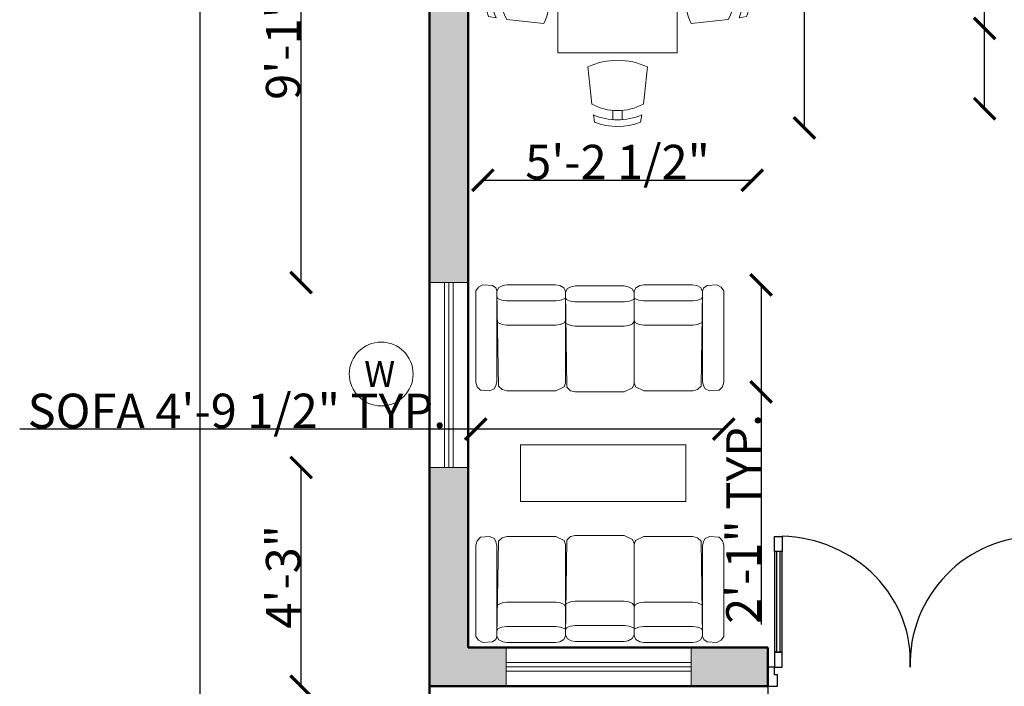
# Model space of a CAD drawing. Units: inches. Extents: x 2169 to 2662, y 1518 to 2151.
# Tile 2 of 6: x 2169 to 2398, y 1596 to 1751. Entities that reach past the tile are written whole.
import ezdxf

# ---------------------------------------------------------------- set-up
doc = ezdxf.new("R2010")
doc.units = ezdxf.units.IN
for name, color, linetype, lineweight in [('A-ANNO-DIMS', 2, 'Continuous', 18), ('A-ANNO-SYMB', 7, 'Continuous', 18), ('A-FURN', 8, 'Continuous', 18), ('A-WALL-PATT', 30, 'Continuous', 13), ('L-PLNT-BEDS', 94, 'Continuous', 25), ('Main Door', 150, 'Continuous', 30), ('Walls', 7, 'Continuous', 50), ('Windows', 160, 'Continuous', 18)]:
    doc.layers.add(name, color=color, linetype=linetype, lineweight=lineweight)
doc.layers.add('A-Glaz', color=92, linetype='Continuous')
doc.styles.get("Standard").update_dxf_attribs({"font": 'arial.ttf'})
doc.dimstyles.get("Standard").update_dxf_attribs({"dimtxt": 8, "dimasz": 5, "dimexe": 0.18, "dimexo": 0.0625, "dimgap": 0.09, "dimtad": 1, "dimdec": 1, "dimzin": 0, "dimdsep": 46, "dimlunit": 4, "dimtxsty": 'Standard', "dimblk": 'ARCHTICK', "dimcen": 0.09, "dimse1": 1, "dimse2": 1, "dimadec": 0, "dimazin": 0, "dimtfac": 1, "dimtdec": 1, "dimtofl": 0, "dimtmove": 0, "dimatfit": 3, "dimfxl": 1, "dimtolj": 1, "dimtzin": 0, "dimarcsym": 0})

# ---------------------------------------------------------------- blocks, each defined once
blk = doc.blocks.new('_ArchTick')
at = {"color": 0, "linetype": 'ByBlock', "const_width": 0.15}
blk.add_lwpolyline([(-0.5, -0.5), (0.5, 0.5)], dxfattribs=at)
blk = doc.blocks.new('*D4')
at = {"layer": 'A-ANNO-DIMS', "color": 0, "lineweight": -2, "transparency": 16777216}
blk.add_line((2210.62, 1555.6), (2210.62, 2111.6), dxfattribs=at)
at = {"layer": 'Defpoints', "color": 0, "transparency": 16777216}
for p in [(2210.62, 2111.6), (2263.98, 2111.6), (2263.98, 1555.6)]:
    blk.add_point(p, dxfattribs=at)
at = {"layer": 'A-ANNO-DIMS', "color": 0, "lineweight": -2, "transparency": 16777216, "xscale": 5, "yscale": 5, "zscale": 5}
for p, rotation in [((2210.62, 2111.6), 90), ((2210.62, 1555.6), 270)]:
    blk.add_blockref('_ArchTick', p, dxfattribs=dict(at, rotation=rotation))
at = {"layer": 'A-ANNO-DIMS', "color": 0, "transparency": 16777216, "insert": (2206.45, 1833.6), "char_height": 8, "attachment_point": 5, "rotation": 90}
blk.add_mtext('\\A1;46\'-4"', dxfattribs=at)
blk = doc.blocks.new('A$C13CE0A17')
at = {"layer": 'A-Glaz'}
for p, q in [((0.01, 0.61), (0.01, 0.08)), ((0.03, 0.08), (0.03, 0.61))]:
    blk.add_line(p, q, dxfattribs=at)
blk.add_lwpolyline([(1.4, 0.08), (1.4, 0.61), (1.42, 0.61), (1.42, 0.08)], close=True, dxfattribs=at)
at = {"layer": 'Main Door'}
for p, q in [((0, 0.61), (0, 0.69)), ((0, 0.69), (0.04, 0.69)), ((0.04, 0.69), (0.04, 0.61)), ((0, 0.61), (0, 0.08)), ((0.04, 0.61), (0, 0.61)), ((0.04, 0.61), (0, 0.61)), ((0.03, 0.61), (0.01, 0.61)), ((0.04, 0.08), (0.04, 0.61)), ((0, 0.08), (0, 0)), ((0.04, 0.08), (0, 0.08)), ((0, 0.08), (0.04, 0.08)), ((0.01, 0.08), (0.03, 0.08)), ((0.04, 0), (0.04, 0.08)), ((-0.035, 0), (-0.035, -0.1)), ((0, 0), (-0.035, 0)), ((0, 0), (0.04, 0)), ((0, -0.04), (0, 0)), ((0.015, -0.04), (0, -0.04)), ((0.015, -0.05), (0.015, -0.04)), ((0.015, -0.1), (0.015, -0.05)), ((-0.035, -0.1), (0.015, -0.1))]:
    blk.add_line(p, q, dxfattribs=at)
for points in [[(1.39, 0.69), (1.39, 0.61), (1.43, 0.61), (1.43, 0.69)], [(1.39, 0.08), (1.39, 0.61), (1.43, 0.61), (1.43, 0.08)], [(1.39, 0), (1.39, 0.08), (1.43, 0.08), (1.43, 0)], [(1.43, 0), (1.465, 0), (1.465, -0.1), (1.415, -0.1), (1.415, -0.05), (1.415, -0.04), (1.43, -0.04)]]:
    blk.add_lwpolyline(points, close=True, dxfattribs=at)
blk.add_arc((1.3872, 0.017), 0.673, 89.7657, 181.4438, dxfattribs=at)
blk.add_ellipse((0.0389, 0.0511), major_axis=(0.6669, -0.1217), ratio=0.940794, start_param=0.11153, end_param=1.73917, dxfattribs=at)
blk = doc.blocks.new('12PCOU17')
at = {"color": 0, "linetype": 'ByBlock'}
for points in [[(-34.71, 34.72), (-33.66, 34.31), (-3.27, 34.3), (-1.81, 34.76), (-1.05, 35.2), (-0.38, 36.65), (-0.61, 39.84), (-1.73, 40.94), (-3.27, 41.4), (-33.66, 41.4), (-34.95, 40.5), (-35.65, 39.02), (-35.49, 35.83), (-34.71, 34.72)], [(-1.89, 11.91), (-1.66, 11.91), (-0.35, 14.68), (-0.35, 31.05), (-0.74, 32.58), (-1.89, 33.83), (-33.63, 34.3), (-34.84, 33.63), (-35.43, 32.38), (-35.68, 31), (-35.68, 14.74), (-35.43, 13.36), (-34.66, 11.99), (-33.44, 11.43), (-3, 11.44), (-1.66, 11.91)], [(-31.25, 11.43), (-31.06, 11.84), (-30.6, 13.09), (-30.4, 14.62), (-30.4, 31.12), (-30.6, 32.65), (-31.06, 33.9), (-31.81, 34.3)], [(-23.84, 11.43), (-22.99, 11.9), (-22.46, 13.15), (-22.23, 14.67), (-22.23, 31.07), (-22.46, 32.59), (-22.99, 33.84), (-23.12, 34.3)], [(-1.54, -10.96), (-1.31, -10.96), (0, -8.19), (0, 8.19), (-0.39, 9.71), (-1.54, 10.96), (-33.28, 11.44), (-34.5, 10.77), (-35.08, 9.51), (-35.33, 8.14), (-35.33, -8.13), (-35.08, -9.51), (-34.31, -10.87), (-33.1, -11.44), (-2.65, -11.43), (-1.31, -10.96)], [(-30.9, -11.44), (-30.72, -11.02), (-30.25, -9.77), (-30.05, -8.25), (-30.05, 8.26), (-30.25, 9.78), (-30.72, 11.03), (-31.47, 11.44)], [(-23.49, -11.44), (-22.64, -10.96), (-22.11, -9.72), (-21.88, -8.19), (-21.88, 8.2), (-22.11, 9.73), (-22.64, 10.97), (-22.77, 11.44)], [(-1.89, -11.91), (-1.66, -11.91), (-0.35, -14.68), (-0.35, -31.05), (-0.74, -32.58), (-1.89, -33.83), (-33.63, -34.3), (-34.84, -33.63), (-35.43, -32.38), (-35.68, -31), (-35.68, -14.74), (-35.43, -13.36), (-34.66, -11.99), (-33.44, -11.43), (-3, -11.44), (-1.66, -11.91)], [(-31.25, -11.43), (-31.06, -11.84), (-30.6, -13.09), (-30.4, -14.62), (-30.4, -31.12), (-30.6, -32.65), (-31.06, -33.9), (-31.81, -34.3)], [(-23.84, -11.43), (-22.99, -11.9), (-22.46, -13.15), (-22.23, -14.67), (-22.23, -31.07), (-22.46, -32.59), (-22.99, -33.84), (-23.12, -34.3)], [(-34.71, -34.72), (-33.66, -34.31), (-3.27, -34.3), (-1.81, -34.76), (-1.05, -35.2), (-0.38, -36.65), (-0.61, -39.84), (-1.73, -40.94), (-3.27, -41.4), (-33.66, -41.4), (-34.95, -40.5), (-35.65, -39.02), (-35.49, -35.83), (-34.71, -34.72)]]:
    blk.add_lwpolyline(points, dxfattribs=at)
blk = doc.blocks.new('table-23')
at = {"color": 0, "linetype": 'ByBlock'}
for p, q in [((-0.6323, 0.4685), (-0.6236, 0.5245)), ((-0.2677, 0.4685), (-0.2764, 0.5245)), ((-0.485, 0.5057), (-0.485, 0.4355)), ((-0.415, 0.5057), (-0.415, 0.4355)), ((-0.675, 0.107), (-0.645, 0.387)), ((-0.225, 0.107), (-0.255, 0.387)), ((-0.9, -1.4923), (-0.9, 0)), ((-0.9, 0), (0, 0)), ((0, -1.4923), (0, 0)), ((-1.0062, -0.2211), (-1.2862, -0.2511)), ((0.1062, -0.2211), (0.3862, -0.2511)), ((-1.3677, -0.2639), (-1.4237, -0.2726)), ((0.4677, -0.2639), (0.5237, -0.2726)), ((-1.4049, -0.4111), (-1.3347, -0.4111)), ((0.5049, -0.4111), (0.4347, -0.4111)), ((-1.4049, -0.4811), (-1.3347, -0.4811)), ((0.5049, -0.4811), (0.4347, -0.4811)), ((-1.3677, -0.6284), (-1.4237, -0.6197)), ((-1.0062, -0.6711), (-1.2862, -0.6411)), ((0.1062, -0.6711), (0.3862, -0.6411)), ((0.4677, -0.6284), (0.5237, -0.6197)), ((-1.3677, -0.8639), (-1.4237, -0.8726)), ((-1.0062, -0.8211), (-1.2862, -0.8511)), ((0.1062, -0.8211), (0.3862, -0.8511)), ((0.4677, -0.8639), (0.5237, -0.8726)), ((-1.4049, -1.0111), (-1.3347, -1.0111)), ((0.5049, -1.0111), (0.4347, -1.0111)), ((-1.4049, -1.0811), (-1.3347, -1.0811)), ((0.5049, -1.0811), (0.4347, -1.0811)), ((-1.3677, -1.2284), (-1.4237, -1.2197)), ((-1.0062, -1.2711), (-1.2862, -1.2411)), ((0.1062, -1.2711), (0.3862, -1.2411)), ((0.4677, -1.2284), (0.5237, -1.2197)), ((-0.9, -1.4923), (0, -1.4923)), ((-0.675, -1.5993), (-0.645, -1.8793)), ((-0.225, -1.5993), (-0.255, -1.8793)), ((-0.485, -1.998), (-0.485, -1.9278)), ((-0.415, -1.998), (-0.415, -1.9278)), ((-0.6323, -1.9608), (-0.6236, -2.0168)), ((-0.2677, -1.9608), (-0.2764, -2.0168))]:
    blk.add_line(p, q, dxfattribs=at)
for centre, radius, start, end in [((-0.45, 0.0773), 0.4797, 68.78869, 111.21131), ((-0.45, 0.0566), 0.4505, 66.13443, 113.86557), ((-0.45, 0.0318), 0.4053, 61.23721, 118.76279), ((-0.45, 0.5883), 0.5312, 244.94238, 295.05762), ((-1.4875, -0.4461), 0.5312, 334.94238, 25.05762), ((0.5875, -0.4461), 0.5312, 154.94238, 205.05762), ((-0.9765, -0.4461), 0.4797, 158.78869, 201.21131), ((-0.9558, -0.4461), 0.4505, 156.13443, 203.86557), ((-0.931, -0.4461), 0.4053, 151.23721, 208.76279), ((0.031, -0.4461), 0.4053, 331.23721, 28.76279), ((0.0558, -0.4461), 0.4505, 336.13443, 23.86557), ((0.0765, -0.4461), 0.4797, 338.78869, 21.21131), ((-0.9765, -1.0461), 0.4797, 158.78869, 201.21131), ((-0.9558, -1.0461), 0.4505, 156.13443, 203.86557), ((-0.931, -1.0461), 0.4053, 151.23721, 208.76279), ((-1.4875, -1.0461), 0.5312, 334.94238, 25.05762), ((0.5875, -1.0461), 0.5312, 154.94238, 205.05762), ((0.031, -1.0461), 0.4053, 331.23721, 28.76279), ((0.0558, -1.0461), 0.4505, 336.13443, 23.86557), ((0.0765, -1.0461), 0.4797, 338.78869, 21.21131), ((-0.45, -2.0806), 0.5312, 64.94238, 115.05762), ((-0.45, -1.5241), 0.4053, 241.23721, 298.76279), ((-0.45, -1.5489), 0.4505, 246.13443, 293.86557), ((-0.45, -1.5696), 0.4797, 248.78869, 291.21131)]:
    blk.add_arc(centre, radius, start, end, dxfattribs=at)
blk = doc.blocks.new('GLAZING-43IN')
for p, q in [((-21.5, 1), (21.5, 1)), ((-21.5, 0), (21.5, 0)), ((-21.5, -1), (21.5, -1))]:
    blk.add_line(p, q)
blk = doc.blocks.new('OPENING-TAG-W')
blk.add_circle((0, 0), 7.42)
blk.add_text('W', height=6).set_placement((-3.96, -3))
blk = doc.blocks.new('*D41')
at = {"layer": 'A-ANNO-DIMS', "color": 0, "lineweight": -2, "transparency": 16777216}
for p, q in [((2342.72, 1585.67), (2408.92, 1585.67)), ((2408.92, 1585.67), (2502.68, 1585.67))]:
    blk.add_line(p, q, dxfattribs=at)
at = {"layer": 'Defpoints', "color": 0, "transparency": 16777216}
for p in [(2342.72, 1595.6), (2408.92, 1595.6), (2408.92, 1585.67)]:
    blk.add_point(p, dxfattribs=at)
at = {"layer": 'A-ANNO-DIMS', "color": 0, "lineweight": -2, "transparency": 16777216, "xscale": 5, "yscale": 5, "zscale": 5, "rotation": 180}
blk.add_blockref('_ArchTick', (2342.72, 1585.67), dxfattribs=at)
at = {"layer": 'A-ANNO-DIMS', "color": 0, "lineweight": -2, "transparency": 16777216, "xscale": 5, "yscale": 5, "zscale": 5}
blk.add_blockref('_ArchTick', (2408.92, 1585.67), dxfattribs=at)
at = {"layer": 'A-ANNO-DIMS', "color": 0, "transparency": 16777216, "insert": (2458.3, 1589.9), "char_height": 8, "attachment_point": 5}
blk.add_mtext('\\A1;MAIN DOOR 5\'-6"', dxfattribs=at)
blk = doc.blocks.new('*D45')
at = {"layer": 'A-ANNO-DIMS', "color": 0, "lineweight": -2, "transparency": 16777216}
for p, q in [((2274.75, 1655.41), (2168.67, 1655.41)), ((2332.47, 1655.41), (2274.75, 1655.41))]:
    blk.add_line(p, q, dxfattribs=at)
at = {"layer": 'Defpoints', "color": 0, "transparency": 16777216}
for p in [(2274.75, 1664.07), (2332.47, 1664.07), (2274.75, 1655.41)]:
    blk.add_point(p, dxfattribs=at)
at = {"layer": 'A-ANNO-DIMS', "color": 0, "lineweight": -2, "transparency": 16777216, "xscale": 5, "yscale": 5, "zscale": 5, "rotation": 180}
blk.add_blockref('_ArchTick', (2274.75, 1655.41), dxfattribs=at)
at = {"layer": 'A-ANNO-DIMS', "color": 0, "lineweight": -2, "transparency": 16777216, "xscale": 5, "yscale": 5, "zscale": 5}
blk.add_blockref('_ArchTick', (2332.47, 1655.41), dxfattribs=at)
at = {"layer": 'A-ANNO-DIMS', "color": 0, "transparency": 16777216, "insert": (2219.21, 1659.64), "char_height": 8, "attachment_point": 5}
blk.add_mtext('\\A1;SOFA 4\'-9 1/2" TYP.', dxfattribs=at)
blk = doc.blocks.new('*D46')
at = {"layer": 'A-ANNO-DIMS', "color": 0, "lineweight": -2, "transparency": 16777216}
for p, q in [((2341.13, 1688.94), (2341.13, 1664.07)), ((2341.13, 1664.07), (2341.13, 1609.99))]:
    blk.add_line(p, q, dxfattribs=at)
at = {"layer": 'Defpoints', "color": 0, "transparency": 16777216}
for p in [(2332.47, 1688.94), (2332.47, 1664.07), (2341.13, 1664.07)]:
    blk.add_point(p, dxfattribs=at)
at = {"layer": 'A-ANNO-DIMS', "color": 0, "lineweight": -2, "transparency": 16777216, "xscale": 5, "yscale": 5, "zscale": 5}
for p, rotation in [((2341.13, 1688.94), 90), ((2341.13, 1664.07), 270)]:
    blk.add_blockref('_ArchTick', p, dxfattribs=dict(at, rotation=rotation))
at = {"layer": 'A-ANNO-DIMS', "color": 0, "transparency": 16777216, "insert": (2337.02, 1634.53), "char_height": 8, "attachment_point": 5, "rotation": 90}
blk.add_mtext('\\A1;2\'-1" TYP.', dxfattribs=at)
blk = doc.blocks.new('*D47')
at = {"layer": 'A-ANNO-DIMS', "color": 0, "lineweight": -2, "transparency": 16777216}
for p, q in [((2351.22, 1806.38), (2351.22, 1899.49)), ((2351.22, 1725.43), (2351.22, 1806.38))]:
    blk.add_line(p, q, dxfattribs=at)
at = {"layer": 'Defpoints', "color": 0, "transparency": 16777216}
for p in [(2339.08, 1806.38), (2351.22, 1806.38), (2339.08, 1725.43)]:
    blk.add_point(p, dxfattribs=at)
at = {"layer": 'A-ANNO-DIMS', "color": 0, "lineweight": -2, "transparency": 16777216, "xscale": 5, "yscale": 5, "zscale": 5}
for p, rotation in [((2351.22, 1806.38), 90), ((2351.22, 1725.43), 270)]:
    blk.add_blockref('_ArchTick', p, dxfattribs=dict(at, rotation=rotation))
at = {"layer": 'A-ANNO-DIMS', "color": 0, "transparency": 16777216, "insert": (2347, 1855.43), "char_height": 8, "attachment_point": 5, "rotation": 90}
blk.add_mtext('\\A1;DINING SET 6\'-9"', dxfattribs=at)
blk = doc.blocks.new('*D48')
at = {"layer": 'A-ANNO-DIMS', "color": 0, "lineweight": -2, "transparency": 16777216}
blk.add_line((2276.42, 1713.29), (2339.08, 1713.29), dxfattribs=at)
at = {"layer": 'Defpoints', "color": 0, "transparency": 16777216}
for p in [(2276.42, 1725.43), (2339.08, 1725.43), (2339.08, 1713.29)]:
    blk.add_point(p, dxfattribs=at)
at = {"layer": 'A-ANNO-DIMS', "color": 0, "lineweight": -2, "transparency": 16777216, "xscale": 5, "yscale": 5, "zscale": 5, "rotation": 180}
blk.add_blockref('_ArchTick', (2276.42, 1713.29), dxfattribs=at)
at = {"layer": 'A-ANNO-DIMS', "color": 0, "lineweight": -2, "transparency": 16777216, "xscale": 5, "yscale": 5, "zscale": 5}
blk.add_blockref('_ArchTick', (2339.08, 1713.29), dxfattribs=at)
at = {"layer": 'A-ANNO-DIMS', "color": 0, "transparency": 16777216, "insert": (2307.75, 1717.51), "char_height": 8, "attachment_point": 5}
blk.add_mtext('\\A1;5\'-2 1/2"', dxfattribs=at)
blk = doc.blocks.new('*D58')
at = {"layer": 'A-ANNO-DIMS', "color": 0, "lineweight": -2, "transparency": 16777216}
blk.add_line((2234.13, 1595.6), (2234.13, 1646.49), dxfattribs=at)
at = {"layer": 'Defpoints', "color": 0, "transparency": 16777216}
for p in [(2234.13, 1646.49), (2263.98, 1646.49), (2263.98, 1595.6)]:
    blk.add_point(p, dxfattribs=at)
at = {"layer": 'A-ANNO-DIMS', "color": 0, "lineweight": -2, "transparency": 16777216, "xscale": 5, "yscale": 5, "zscale": 5}
for p, rotation in [((2234.13, 1646.49), 90), ((2234.13, 1595.6), 270)]:
    blk.add_blockref('_ArchTick', p, dxfattribs=dict(at, rotation=rotation))
at = {"layer": 'A-ANNO-DIMS', "color": 0, "transparency": 16777216, "insert": (2229.95, 1621.05), "char_height": 8, "attachment_point": 5, "rotation": 90}
blk.add_mtext('\\A1;4\'-3"', dxfattribs=at)
blk = doc.blocks.new('*D59')
at = {"layer": 'A-ANNO-DIMS', "color": 0, "lineweight": -2, "transparency": 16777216}
blk.add_line((2234.13, 1689.49), (2234.13, 1798.55), dxfattribs=at)
at = {"layer": 'Defpoints', "color": 0, "transparency": 16777216}
for p in [(2234.13, 1798.55), (2263.98, 1798.55), (2263.98, 1689.49)]:
    blk.add_point(p, dxfattribs=at)
at = {"layer": 'A-ANNO-DIMS', "color": 0, "lineweight": -2, "transparency": 16777216, "xscale": 5, "yscale": 5, "zscale": 5}
for p, rotation in [((2234.13, 1798.55), 90), ((2234.13, 1689.49), 270)]:
    blk.add_blockref('_ArchTick', p, dxfattribs=dict(at, rotation=rotation))
at = {"layer": 'A-ANNO-DIMS', "color": 0, "transparency": 16777216, "insert": (2229.95, 1744.02), "char_height": 8, "attachment_point": 5, "rotation": 90}
blk.add_mtext('\\A1;9\'-1"', dxfattribs=at)
blk = doc.blocks.new('*D70')
at = {"layer": 'A-ANNO-DIMS', "color": 0, "lineweight": -2, "transparency": 16777216}
blk.add_line((2272.98, 1525.75), (2370.48, 1525.75), dxfattribs=at)
at = {"layer": 'Defpoints', "color": 0, "transparency": 16777216}
for p in [(2272.98, 1886.6), (2370.48, 1886.6), (2370.48, 1525.75)]:
    blk.add_point(p, dxfattribs=at)
at = {"layer": 'A-ANNO-DIMS', "color": 0, "lineweight": -2, "transparency": 16777216, "xscale": 5, "yscale": 5, "zscale": 5, "rotation": 180}
blk.add_blockref('_ArchTick', (2272.98, 1525.75), dxfattribs=at)
at = {"layer": 'A-ANNO-DIMS', "color": 0, "lineweight": -2, "transparency": 16777216, "xscale": 5, "yscale": 5, "zscale": 5}
blk.add_blockref('_ArchTick', (2370.48, 1525.75), dxfattribs=at)
at = {"layer": 'A-ANNO-DIMS', "color": 0, "transparency": 16777216, "insert": (2321.73, 1529.98), "char_height": 8, "attachment_point": 5}
blk.add_mtext('\\A1;8\'-1 1/2"', dxfattribs=at)
blk = doc.blocks.new('*D71')
at = {"layer": 'A-ANNO-DIMS', "color": 0, "lineweight": -2, "transparency": 16777216}
for p, q in [((2300.48, 1525.75), (2310.48, 1525.75)), ((2310.48, 1525.75), (2343.14, 1525.75))]:
    blk.add_line(p, q, dxfattribs=at)
at = {"layer": 'Defpoints', "color": 0, "transparency": 16777216}
for p in [(2300.48, 1886.6), (2310.48, 1886.6), (2310.48, 1525.75)]:
    blk.add_point(p, dxfattribs=at)
at = {"layer": 'A-ANNO-DIMS', "color": 0, "lineweight": -2, "transparency": 16777216, "xscale": 5, "yscale": 5, "zscale": 5, "rotation": 180}
blk.add_blockref('_ArchTick', (2300.48, 1525.75), dxfattribs=at)
at = {"layer": 'A-ANNO-DIMS', "color": 0, "lineweight": -2, "transparency": 16777216, "xscale": 5, "yscale": 5, "zscale": 5}
blk.add_blockref('_ArchTick', (2310.48, 1525.75), dxfattribs=at)
at = {"layer": 'A-ANNO-DIMS', "color": 0, "transparency": 16777216, "insert": (2329.31, 1529.93), "char_height": 8, "attachment_point": 5}
blk.add_mtext('\\A1;0\'-10"', dxfattribs=at)
blk = doc.blocks.new('*D74')
at = {"layer": 'A-ANNO-DIMS', "color": 0, "lineweight": -2, "transparency": 16777216}
for p, q in [((2272.98, 1525.75), (2300.48, 1525.75)), ((2300.48, 1525.75), (2345.7, 1525.75))]:
    blk.add_line(p, q, dxfattribs=at)
at = {"layer": 'Defpoints', "color": 0, "transparency": 16777216}
for p in [(2272.98, 1886.6), (2300.48, 1886.6), (2300.48, 1525.75)]:
    blk.add_point(p, dxfattribs=at)
at = {"layer": 'A-ANNO-DIMS', "color": 0, "lineweight": -2, "transparency": 16777216, "xscale": 5, "yscale": 5, "zscale": 5, "rotation": 180}
blk.add_blockref('_ArchTick', (2272.98, 1525.75), dxfattribs=at)
at = {"layer": 'A-ANNO-DIMS', "color": 0, "lineweight": -2, "transparency": 16777216, "xscale": 5, "yscale": 5, "zscale": 5}
blk.add_blockref('_ArchTick', (2300.48, 1525.75), dxfattribs=at)
at = {"layer": 'A-ANNO-DIMS', "color": 0, "transparency": 16777216, "insert": (2325.59, 1529.98), "char_height": 8, "attachment_point": 5}
blk.add_mtext('\\A1;2\'-3 1/2"', dxfattribs=at)
blk = doc.blocks.new('*D78')
at = {"layer": 'A-ANNO-DIMS', "color": 0, "lineweight": -2, "transparency": 16777216}
for p, q in [((2393.13, 1748.6), (2393.13, 1792.94)), ((2393.13, 1729.93), (2393.13, 1748.6))]:
    blk.add_line(p, q, dxfattribs=at)
at = {"layer": 'Defpoints', "color": 0, "transparency": 16777216}
for p in [(2393.13, 1748.6), (2422.98, 1748.6), (2422.98, 1729.93)]:
    blk.add_point(p, dxfattribs=at)
at = {"layer": 'A-ANNO-DIMS', "color": 0, "lineweight": -2, "transparency": 16777216, "xscale": 5, "yscale": 5, "zscale": 5}
for p, rotation in [((2393.13, 1748.6), 90), ((2393.13, 1729.93), 270)]:
    blk.add_blockref('_ArchTick', p, dxfattribs=dict(at, rotation=rotation))
at = {"layer": 'A-ANNO-DIMS', "color": 0, "transparency": 16777216, "insert": (2388.9, 1773.27), "char_height": 8, "attachment_point": 5, "rotation": 90}
blk.add_mtext('\\A1;1\'-6 1/2"', dxfattribs=at)
blk = doc.blocks.new('*D80')
at = {"layer": 'A-ANNO-DIMS', "color": 0, "lineweight": -2, "transparency": 16777216}
for p, q in [((2285.18, 1525.75), (2323.65, 1525.75)), ((2323.65, 1525.75), (2368.73, 1525.75))]:
    blk.add_line(p, q, dxfattribs=at)
at = {"layer": 'Defpoints', "color": 0, "transparency": 16777216}
for p in [(2285.18, 1638.55), (2323.65, 1638.55), (2323.65, 1525.75)]:
    blk.add_point(p, dxfattribs=at)
at = {"layer": 'A-ANNO-DIMS', "color": 0, "lineweight": -2, "transparency": 16777216, "xscale": 5, "yscale": 5, "zscale": 5, "rotation": 180}
blk.add_blockref('_ArchTick', (2285.18, 1525.75), dxfattribs=at)
at = {"layer": 'A-ANNO-DIMS', "color": 0, "lineweight": -2, "transparency": 16777216, "xscale": 5, "yscale": 5, "zscale": 5}
blk.add_blockref('_ArchTick', (2323.65, 1525.75), dxfattribs=at)
at = {"layer": 'A-ANNO-DIMS', "color": 0, "transparency": 16777216, "insert": (2348.69, 1529.98), "char_height": 8, "attachment_point": 5}
blk.add_mtext('\\A1;3\'-2 1/2"', dxfattribs=at)
blk = doc.blocks.new('*D81')
at = {"layer": 'A-ANNO-DIMS', "color": 0, "lineweight": -2, "transparency": 16777216}
for p, q in [((2624.02, 1651.77), (2624.02, 1677.47)), ((2624.02, 1638.55), (2624.02, 1651.77))]:
    blk.add_line(p, q, dxfattribs=at)
at = {"layer": 'Defpoints', "color": 0, "transparency": 16777216}
for p in [(2323.65, 1651.77), (2624.02, 1651.77), (2323.65, 1638.55)]:
    blk.add_point(p, dxfattribs=at)
at = {"layer": 'A-ANNO-DIMS', "color": 0, "lineweight": -2, "transparency": 16777216, "xscale": 5, "yscale": 5, "zscale": 5}
for p, rotation in [((2624.02, 1651.77), 90), ((2624.02, 1638.55), 270)]:
    blk.add_blockref('_ArchTick', p, dxfattribs=dict(at, rotation=rotation))
at = {"layer": 'A-ANNO-DIMS', "color": 0, "transparency": 16777216, "insert": (2619.91, 1667.12), "char_height": 8, "attachment_point": 5, "rotation": 90}
blk.add_mtext('\\A1;1\'-1"', dxfattribs=at)

msp = doc.modelspace()

# ---------------------------------------------------------------- hatches: boundary and pattern name
at = {"layer": 'A-WALL-PATT', "transparency": 33554585}
h = msp.add_hatch(color=256, dxfattribs=at)
h.dxf.hatch_style = 1
h.paths.add_polyline_path([(2575.98, 2111.6), (2263.98, 2111.6), (2263.98, 2066.68), (2272.98, 2066.68), (2272.98, 2102.6), (2418.98, 2102.6), (2418.98, 1982.6), (2413.75, 1982.6), (2413.75, 1978.6), (2418.98, 1978.6), (2418.98, 1954.6), (2429.26, 1954.6), (2429.26, 1958.6), (2422.98, 1958.6), (2422.98, 2102.6), (2566.98, 2102.6), (2566.98, 2052.1), (2575.98, 2052.1)])
h.paths.add_polyline_path([(2575.98, 2009.1), (2566.98, 2009.1), (2566.98, 1997.84), (2566.98, 1958.6), (2467.98, 1958.6), (2467.98, 1950.67), (2471.98, 1950.67), (2471.98, 1954.6), (2566.98, 1954.6), (2566.98, 1947.83), (2575.98, 1947.83)])
h.paths.add_polyline_path([(2272.98, 2023.68), (2263.98, 2023.68), (2263.98, 1944.7), (2272.98, 1944.7), (2272.98, 1978.6), (2369.77, 1978.6), (2369.77, 1982.6), (2272.98, 1982.6)])
h.paths.add_polyline_path([(2272.98, 1882.6), (2370.48, 1882.6), (2370.48, 1886.6), (2272.98, 1886.6), (2272.98, 1921.26), (2263.98, 1921.26), (2263.98, 1841.55), (2272.98, 1841.55)])
h.paths.add_polyline_path([(2272.98, 1798.55), (2263.98, 1798.55), (2263.98, 1689.49), (2272.98, 1689.49)])
h.paths.add_polyline_path([(2272.98, 1646.49), (2263.98, 1646.49), (2263.98, 1595.6), (2281.85, 1595.6), (2281.85, 1604.6), (2272.98, 1604.6)])
h.paths.add_polyline_path([(2342.72, 1600.02), (2342.72, 1604.6), (2324.85, 1604.6), (2324.85, 1595.6), (2342.72, 1595.6)])
h.paths.add_polyline_path([(2462.45, 1604.6), (2408.92, 1604.6), (2408.92, 1595.6), (2462.45, 1595.6)])
h.paths.add_polyline_path([(2422.98, 1689.75), (2418.98, 1689.75), (2418.98, 1604.6), (2422.98, 1604.6)])
h.paths.add_polyline_path([(2575.98, 1655.1), (2566.98, 1655.1), (2566.98, 1643.84), (2566.98, 1604.6), (2522.45, 1604.6), (2522.45, 1595.6), (2575.98, 1595.6)])
h.paths.add_polyline_path([(2575.98, 1791.1), (2566.98, 1791.1), (2566.98, 1752.6), (2422.98, 1752.6), (2422.98, 1816.31), (2418.98, 1816.31), (2418.98, 1729.93), (2422.98, 1729.93), (2422.98, 1748.6), (2566.98, 1748.6), (2566.98, 1698.1), (2575.98, 1698.1)])
h.paths.add_polyline_path([(2575.98, 1883.38), (2566.98, 1883.38), (2566.98, 1876.6), (2506.75, 1876.6), (2506.75, 1872.6), (2566.98, 1872.6), (2566.98, 1834.1), (2575.98, 1834.1)])
h.paths.add_polyline_path([(2477.81, 1876.6), (2471.98, 1876.6), (2471.98, 1913.6), (2566.98, 1913.6), (2566.98, 1906.83), (2575.98, 1906.83), (2575.98, 1924.38), (2566.98, 1924.38), (2566.98, 1917.6), (2471.98, 1917.6), (2471.98, 1921.14), (2467.98, 1921.14), (2467.98, 1876.6), (2418.98, 1876.6), (2418.98, 1855.49), (2422.98, 1855.49), (2422.98, 1872.6), (2477.81, 1872.6)])

# ---------------------------------------------------------------- linework, layer by layer
at = {"layer": 'A-FURN'}
msp.add_lwpolyline([(2285.18, 1651.77), (2323.65, 1651.77), (2323.65, 1638.55), (2285.18, 1638.55)], close=True, dxfattribs=at)
at = {"layer": 'L-PLNT-BEDS'}
msp.add_line((2342.72, 1595.6), (2342.72, 1555.6), dxfattribs=at)
at = {"layer": 'Walls'}
for p, q in [((2263.98, 2111.6), (2263.98, 1555.6)), ((2272.98, 1882.6), (2272.98, 1604.6)), ((2272.98, 1604.6), (2342.72, 1604.6)), ((2342.72, 1604.6), (2342.72, 1595.6)), ((2263.98, 1595.6), (2342.72, 1595.6))]:
    msp.add_line(p, q, dxfattribs=at)
at = {"layer": 'Windows'}
for points in [[(2263.98, 1646.49), (2263.98, 1689.49), (2272.98, 1689.49), (2272.98, 1646.49)], [(2281.85, 1604.6), (2324.85, 1604.6), (2324.85, 1595.6), (2281.85, 1595.6)]]:
    msp.add_lwpolyline(points, close=True, dxfattribs=at)

# ---------------------------------------------------------------- block references
at = {"layer": 'A-ANNO-SYMB'}
msp.add_blockref('OPENING-TAG-W', (2252.77, 1668.23), dxfattribs=at)
at = {"layer": 'A-FURN', "xscale": 30.80298432698044, "yscale": 30.80298432698044, "zscale": 30.80298432698044}
msp.add_blockref('table-23', (2321.61, 1788.89), dxfattribs=at)
at = {"layer": 'A-FURN', "yscale": 0.6971861638371055, "zscale": 0.6971861638371055, "rotation": 90}
for p, xscale in [((2303.61, 1664.07), -0.6971861638371055), ((2303.61, 1630.67), 0.6971861638371055)]:
    msp.add_blockref('12PCOU17', p, dxfattribs=dict(at, xscale=xscale))
at = {"layer": 'Main Door', "xscale": 44.13700514456166, "yscale": 44.13700514456166, "zscale": 44.13700514456166}
msp.add_blockref('A$C13CE0A17', (2344.26, 1600.02), dxfattribs=at)
at = {"layer": 'Windows', "rotation": 89.99999999999991}
msp.add_blockref('GLAZING-43IN', (2268.48, 1667.99), dxfattribs=at)
at = {"layer": 'Windows'}
msp.add_blockref('GLAZING-43IN', (2303.35, 1600.1), dxfattribs=at)

# ---------------------------------------------------------------- dimensions: what is measured, and where the dimension line sits
at = {"layer": 'A-ANNO-DIMS'}
for base, p1, p2, override, picture, middle in [((2210.62, 2111.6), (2263.98, 1555.6), (2263.98, 2111.6), {"dimclrd": 0, "dimclre": 0, "dimclrt": 0}, '*D4', (2206.45, 1833.6)), ((2234.13, 1798.55), (2263.98, 1689.49), (2263.98, 1798.55), {"dimdec": 1, "dimlfac": 1, "dimrnd": 0, "dimzin": 1, "dimdsep": 46, "dimlunit": 4, "dimfrac": 2}, '*D59', (2229.95, 1744.02)), ((2393.13, 1748.6), (2422.98, 1729.93), (2422.98, 1748.6), {"dimdec": 1, "dimlfac": 1, "dimrnd": 0, "dimzin": 1, "dimdsep": 46, "dimlunit": 4, "dimfrac": 2}, '*D78', (2388.9, 1773.27)), ((2624.02, 1651.77), (2323.65, 1638.55), (2323.65, 1651.77), {"dimdec": 1, "dimlfac": 1, "dimrnd": 0, "dimzin": 1, "dimdsep": 46, "dimlunit": 4, "dimfrac": 2}, '*D81', (2619.91, 1667.12)), ((2234.13, 1646.49), (2263.98, 1595.6), (2263.98, 1646.49), {"dimdec": 1, "dimlfac": 1, "dimrnd": 0, "dimzin": 1, "dimdsep": 46, "dimlunit": 4, "dimfrac": 2}, '*D58', (2229.95, 1621.05))]:
    dim = msp.add_linear_dim(base=base, p1=p1, p2=p2, angle=90, dimstyle='Standard', override=override, dxfattribs=at)
    dim.commit()
    dim.dimension.update_dxf_attribs({"geometry": picture, "text_midpoint": middle})
for base, p1, p2, angle, text, picture, middle in [((2351.2225, 1806.38), (2339.0798, 1725.4288), (2339.0798, 1806.38), 90, 'DINING SET <>', '*D47', (2346.9961, 1855.4345)), ((2341.13, 1664.07), (2332.47, 1688.94), (2332.47, 1664.07), 270, '<> TYP.', '*D46', (2337.02, 1634.53)), ((2274.75, 1655.41), (2332.47, 1664.07), (2274.75, 1664.07), 180, 'SOFA <> TYP.', '*D45', (2219.21, 1659.64))]:
    dim = msp.add_linear_dim(base=base, p1=p1, p2=p2, angle=angle, text=text, dimstyle='Standard', override={"dimdec": 1, "dimlfac": 1, "dimrnd": 0, "dimzin": 1, "dimdsep": 46, "dimlunit": 4, "dimfrac": 2}, dxfattribs=at)
    dim.commit()
    dim.dimension.update_dxf_attribs({"geometry": picture, "text_midpoint": middle})
for base, p1, p2, picture, middle in [((2370.48, 1525.75), (2272.98, 1886.6), (2370.48, 1886.6), '*D70', (2321.73, 1529.98)), ((2300.48, 1525.75), (2272.98, 1886.6), (2300.48, 1886.6), '*D74', (2325.59, 1529.98)), ((2310.48, 1525.75), (2300.48, 1886.6), (2310.48, 1886.6), '*D71', (2329.31, 1529.93)), ((2339.08, 1713.29), (2276.42, 1725.43), (2339.08, 1725.43), '*D48', (2307.75, 1717.51)), ((2323.65, 1525.75), (2285.18, 1638.55), (2323.65, 1638.55), '*D80', (2348.69, 1529.98))]:
    dim = msp.add_linear_dim(base=base, p1=p1, p2=p2, dimstyle='Standard', override={"dimdec": 1, "dimlfac": 1, "dimrnd": 0, "dimzin": 1, "dimdsep": 46, "dimlunit": 4, "dimfrac": 2}, dxfattribs=at)
    dim.commit()
    dim.dimension.update_dxf_attribs({"geometry": picture, "text_midpoint": middle})
dim = msp.add_linear_dim(base=(2408.92, 1585.67), p1=(2342.72, 1595.6), p2=(2408.92, 1595.6), text='MAIN DOOR <>', dimstyle='Standard', override={"dimdec": 1, "dimlfac": 1, "dimrnd": 0, "dimzin": 1, "dimdsep": 46, "dimlunit": 4, "dimfrac": 2}, dxfattribs=at)
dim.commit()
dim.dimension.update_dxf_attribs({"geometry": '*D41', "text_midpoint": (2458.3, 1589.9)})

doc.saveas('drawing.dxf')
